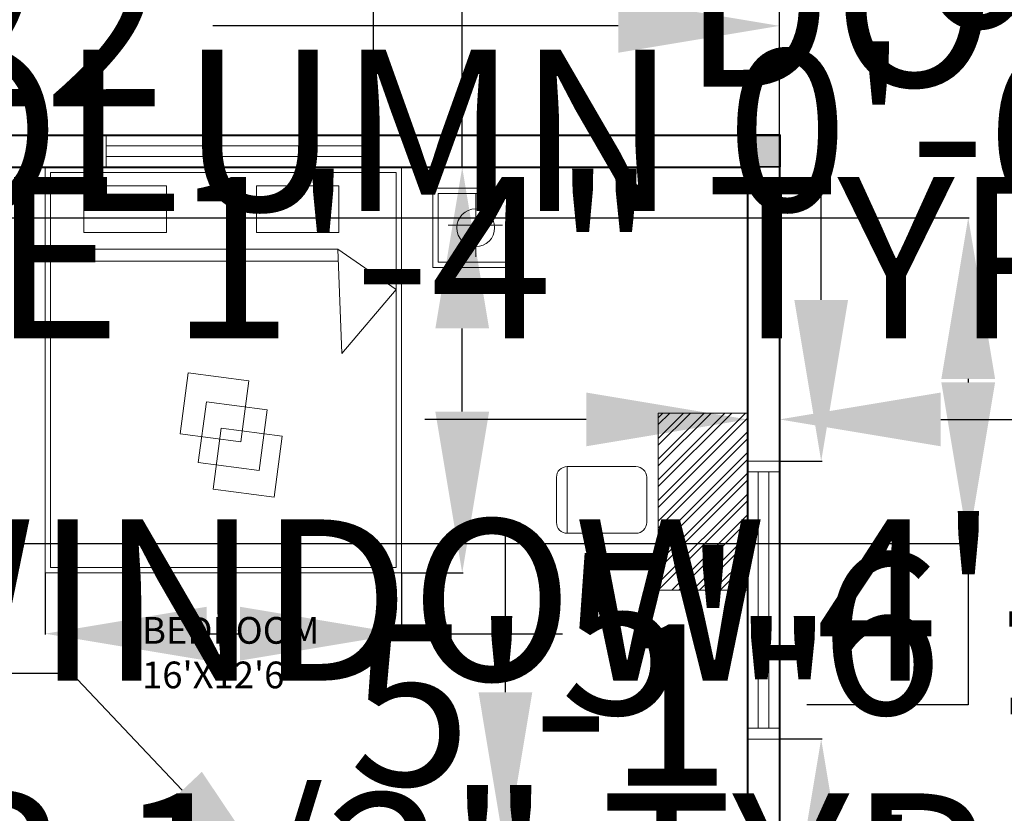
# Model space of a CAD drawing. Units: inches. Extents: x 7323 to 9737, y 2037 to 3322.
# Tile 15 of 19: x 9130 to 9314, y 2560 to 2709. Entities that reach past the tile are written whole.
import ezdxf

# ---------------------------------------------------------------- set-up
doc = ezdxf.new("R2010")
doc.units = ezdxf.units.IN
doc.header["$MEASUREMENT"] = 0
for name, color, linetype, lineweight in [('A-ANNO-DIMS', 2, 'Continuous', 18), ('A-AREA-IDEN', 7, 'Continuous', 18), ('A-COLS', 1, 'Continuous', 35), ('A-FURN', 8, 'Continuous', 18), ('A-FURN-PATT', 252, 'Continuous', 13), ('A-GLAZ', 4, 'Continuous', 18), ('A-WALL', 7, 'Continuous', 40)]:
    doc.layers.add(name, color=color, linetype=linetype, lineweight=lineweight)
doc.layers.add('A-COLS-PATT', color=18, linetype='Continuous', lineweight=13, true_color=0x000000)
doc.styles.get("Standard").update_dxf_attribs({"font": 'arial.ttf'})
doc.dimstyles.get("Standard").update_dxf_attribs({"dimtxt": 30.18, "dimasz": 30.18, "dimexe": 0.18, "dimexo": 0.0625, "dimgap": 0.09, "dimtad": 0, "dimtih": 1, "dimtoh": 1, "dimdec": 0, "dimzin": 0, "dimdsep": 46, "dimlunit": 3, "dimtxsty": 'Standard', "dimcen": 0.09, "dimadec": 0, "dimazin": 0, "dimtfac": 1, "dimtdec": 0, "dimtofl": 0, "dimtmove": 0, "dimatfit": 3, "dimfxl": 1, "dimtolj": 1, "dimtzin": 0, "dimarcsym": 0})

# ---------------------------------------------------------------- blocks, each defined once
blk = doc.blocks.new('*D10')
at = {"layer": 'A-ANNO-DIMS', "color": 0, "lineweight": -2, "transparency": 16777216}
for p, q in [((9007.95, 2687.36), (9007.95, 2707.94)), ((9038.13, 2707.76), (9113.99, 2707.76)), ((9241.77, 2707.76), (9165.9, 2707.76)), ((9271.95, 2687.36), (9271.95, 2707.94))]:
    blk.add_line(p, q, dxfattribs=at)
at = {"layer": 'A-ANNO-DIMS', "color": 0, "transparency": 16777216}
for points in [[(9038.13, 2712.79), (9038.13, 2702.73), (9007.95, 2707.76)], [(9241.77, 2712.79), (9241.77, 2702.73), (9271.95, 2707.76)]]:
    blk.add_solid(points, dxfattribs=at)
at = {"layer": 'Defpoints', "color": 0, "transparency": 16777216}
for p in [(9271.95, 2707.76), (9007.95, 2687.3), (9271.95, 2687.3)]:
    blk.add_point(p, dxfattribs=at)
at = {"layer": 'A-ANNO-DIMS', "color": 0, "transparency": 16777216, "insert": (9139.95, 2707.76), "char_height": 30.18, "attachment_point": 5}
blk.add_mtext("\\A1;22'", dxfattribs=at)
blk = doc.blocks.new('WIN-48')
for p, q in [((0, 0), (0, 6)), ((2, 0), (2, 6)), ((50, 0), (50, 6)), ((52, 0), (52, 6)), ((2, 4), (50, 4)), ((2, 2), (50, 2))]:
    blk.add_line(p, q)
blk = doc.blocks.new('BED-DOUBLE-REAR')
for p, q in [((1, 60.58), (54.75, 60.58)), ((54.75, 60.58), (65.65, 53.04)), ((55.5, 41.06), (54.75, 60.58)), ((54.83, 58.32), (1, 58.32)), ((65.65, 53.04), (55.5, 41.06))]:
    blk.add_line(p, q)
for points in [[(0, 75.91), (66.65, 75.91), (66.65, 0), (0, 0)], [(1, 74.91), (65.65, 74.91), (65.65, 1), (1, 1)], [(7.24, 72.42), (22.67, 72.42), (22.67, 63.7), (7.24, 63.7)], [(39.52, 72.42), (54.95, 72.42), (54.95, 63.7), (39.52, 63.7)], [(36.59, 24.55), (38.1, 35.92), (26.73, 37.42), (25.22, 26.05)], [(40.02, 19.16), (41.52, 30.53), (30.15, 32.04), (28.64, 20.66)], [(42.82, 14.19), (44.32, 25.56), (32.95, 27.06), (31.44, 15.69)]]:
    blk.add_lwpolyline(points, close=True)
blk = doc.blocks.new('BEDSIDE-TABLE-LARGE')
for p, q in [((8.01, 13.84), (8.01, 1.98)), ((2.84, 7.91), (13.05, 7.91))]:
    blk.add_line(p, q)
for points in [[(0, 14.84), (16.03, 14.84), (16.03, 0), (0, 0)], [(1, 13.84), (15.03, 13.84), (15.03, 1), (1, 1)]]:
    blk.add_lwpolyline(points, close=True)
blk.add_circle((8.01, 7.42), 3.54)
blk = doc.blocks.new('COL-PLAN-6IN')
blk.add_lwpolyline([(0, 6), (0, 6), (6.06, 6), (6.06, 6), (6.06, 0), (6.06, 0), (0, 0), (0, 0)], close=True)
blk = doc.blocks.new('*D35')
at = {"layer": 'A-ANNO-DIMS', "color": 0, "lineweight": -2, "transparency": 16777216}
for p, q in [((8977.7, 2688.2), (8947.52, 2688.2)), ((9007.88, 2687.36), (9007.88, 2688.38)), ((9013.95, 2687.36), (9013.95, 2688.38)), ((9044.13, 2688.2), (9074.31, 2688.2))]:
    blk.add_line(p, q, dxfattribs=at)
at = {"layer": 'A-ANNO-DIMS', "color": 0, "transparency": 16777216}
for points in [[(8977.7, 2693.23), (8977.7, 2683.17), (9007.88, 2688.2)], [(9044.13, 2693.23), (9044.13, 2683.17), (9013.95, 2688.2)]]:
    blk.add_solid(points, dxfattribs=at)
at = {"layer": 'Defpoints', "color": 0, "transparency": 16777216}
for p in [(9007.88, 2687.3), (9013.95, 2688.2), (9013.95, 2687.3)]:
    blk.add_point(p, dxfattribs=at)
at = {"layer": 'A-ANNO-DIMS', "color": 0, "transparency": 16777216, "insert": (9263.41, 2688.2), "char_height": 30.18, "attachment_point": 5}
blk.add_mtext('\\A1;COLUMN 0\'-6" TYP.', dxfattribs=at)
blk = doc.blocks.new('*D36')
at = {"layer": 'A-ANNO-DIMS', "color": 0, "lineweight": -2, "transparency": 16777216}
for p, q in [((9006.97, 2717.48), (9006.97, 2747.66)), ((9006.97, 2747.66), (9037.15, 2747.66)), ((9007.82, 2687.3), (9006.79, 2687.3)), ((9007.82, 2681.3), (9006.79, 2681.3)), ((9006.97, 2651.12), (9006.97, 2620.94))]:
    blk.add_line(p, q, dxfattribs=at)
at = {"layer": 'A-ANNO-DIMS', "color": 0, "transparency": 16777216}
for points in [[(9001.94, 2717.48), (9012, 2717.48), (9006.97, 2687.3)], [(9001.94, 2651.12), (9012, 2651.12), (9006.97, 2681.3)]]:
    blk.add_solid(points, dxfattribs=at)
at = {"layer": 'Defpoints', "color": 0, "transparency": 16777216}
for p in [(9006.97, 2687.3), (9007.88, 2687.3), (9007.88, 2681.3)]:
    blk.add_point(p, dxfattribs=at)
at = {"layer": 'A-ANNO-DIMS', "color": 0, "transparency": 16777216, "insert": (9129.22, 2747.66), "char_height": 30.18, "attachment_point": 5}
blk.add_mtext('\\A1;0\'-6" TYP.', dxfattribs=at)
blk = doc.blocks.new('*D37')
at = {"layer": 'A-ANNO-DIMS', "color": 0, "lineweight": -2, "transparency": 16777216}
for p, q in [((9279.75, 2656.48), (9279.75, 2686.66)), ((9272.01, 2626.3), (9279.93, 2626.3)), ((9272.01, 2574.3), (9279.93, 2574.3)), ((9279.75, 2544.12), (9279.75, 2513.94))]:
    blk.add_line(p, q, dxfattribs=at)
at = {"layer": 'A-ANNO-DIMS', "color": 0, "transparency": 16777216}
for points in [[(9274.72, 2656.48), (9284.78, 2656.48), (9279.75, 2626.3)], [(9274.72, 2544.12), (9284.78, 2544.12), (9279.75, 2574.3)]]:
    blk.add_solid(points, dxfattribs=at)
at = {"layer": 'Defpoints', "color": 0, "transparency": 16777216}
for p in [(9271.95, 2626.3), (9271.95, 2574.3), (9279.75, 2574.3)]:
    blk.add_point(p, dxfattribs=at)
at = {"layer": 'A-ANNO-DIMS', "color": 0, "transparency": 16777216, "insert": (9279.75, 2600.3), "char_height": 30.18, "attachment_point": 5}
blk.add_mtext('\\A1;WINDOW 4\'-4" TYP.', dxfattribs=at)
blk = doc.blocks.new('*D38')
at = {"layer": 'A-ANNO-DIMS', "color": 0, "lineweight": -2, "transparency": 16777216}
for p, q in [((9235.77, 2634.1), (9205.59, 2634.1)), ((9265.95, 2626.36), (9265.95, 2634.28)), ((9271.95, 2626.36), (9271.95, 2634.28)), ((9302.13, 2634.1), (9332.31, 2634.1))]:
    blk.add_line(p, q, dxfattribs=at)
at = {"layer": 'A-ANNO-DIMS', "color": 0, "transparency": 16777216}
for points in [[(9235.77, 2639.13), (9235.77, 2629.07), (9265.95, 2634.1)], [(9302.13, 2639.13), (9302.13, 2629.07), (9271.95, 2634.1)]]:
    blk.add_solid(points, dxfattribs=at)
at = {"layer": 'Defpoints', "color": 0, "transparency": 16777216}
for p in [(9271.95, 2634.1), (9265.95, 2626.3), (9271.95, 2626.3)]:
    blk.add_point(p, dxfattribs=at)
at = {"layer": 'A-ANNO-DIMS', "color": 0, "transparency": 16777216, "insert": (9424.38, 2634.1), "char_height": 30.18, "attachment_point": 5}
blk.add_mtext('\\A1;0\'-6" TYP.', dxfattribs=at)
blk = doc.blocks.new('*D39')
at = {"layer": 'A-ANNO-DIMS', "color": 0, "lineweight": -2, "transparency": 16777216}
for p, q in [((8647.94, 2549.03), (8617.76, 2549.03)), ((8678.12, 2543.2), (8678.12, 2549.21)), ((8717.39, 2543.2), (8717.39, 2549.21)), ((8747.57, 2549.03), (8777.75, 2549.03))]:
    blk.add_line(p, q, dxfattribs=at)
at = {"layer": 'A-ANNO-DIMS', "color": 0, "transparency": 16777216}
for points in [[(8647.94, 2554.06), (8647.94, 2544), (8678.12, 2549.03)], [(8747.57, 2554.06), (8747.57, 2544), (8717.39, 2549.03)]]:
    blk.add_solid(points, dxfattribs=at)
at = {"layer": 'Defpoints', "color": 0, "transparency": 16777216}
for p in [(8717.39, 2549.03), (8678.12, 2543.14), (8717.39, 2543.14)]:
    blk.add_point(p, dxfattribs=at)
at = {"layer": 'A-ANNO-DIMS', "color": 0, "transparency": 16777216, "insert": (9057.19, 2549.03), "char_height": 30.18, "attachment_point": 5}
blk.add_mtext('\\A1;SINGLE DOOR 3\'-3 1/2" TYP.', dxfattribs=at)
blk = doc.blocks.new('*D45')
at = {"layer": 'A-ANNO-DIMS', "color": 0, "lineweight": -2, "transparency": 16777216}
for p, q in [((8725.79, 2664.36), (8695.61, 2664.36)), ((8755.97, 2662.02), (8755.97, 2664.54)), ((8772, 2662.02), (8772, 2664.54)), ((8802.18, 2664.36), (8832.36, 2664.36))]:
    blk.add_line(p, q, dxfattribs=at)
at = {"layer": 'A-ANNO-DIMS', "color": 0, "transparency": 16777216}
for points in [[(8725.79, 2669.39), (8725.79, 2659.33), (8755.97, 2664.36)], [(8802.18, 2669.39), (8802.18, 2659.33), (8772, 2664.36)]]:
    blk.add_solid(points, dxfattribs=at)
at = {"layer": 'Defpoints', "color": 0, "transparency": 16777216}
for p in [(8772, 2664.36), (8755.97, 2661.96), (8772, 2661.96)]:
    blk.add_point(p, dxfattribs=at)
at = {"layer": 'A-ANNO-DIMS', "color": 0, "transparency": 16777216, "insert": (9094.8, 2664.36), "char_height": 30.18, "attachment_point": 5}
blk.add_mtext('\\A1;BEDSIDE TABLE 1\'-4" TYP.', dxfattribs=at)
blk = doc.blocks.new('*D51')
at = {"layer": 'A-ANNO-DIMS', "color": 0, "lineweight": -2, "transparency": 16777216}
for p, q in [((9130.95, 2513.23), (9130.95, 2501.42)), ((9208.95, 2513.23), (9208.95, 2501.42)), ((9161.13, 2501.6), (9178.77, 2501.6)), ((9208.95, 2501.6), (9239.13, 2501.6))]:
    blk.add_line(p, q, dxfattribs=at)
at = {"layer": 'A-ANNO-DIMS', "color": 0, "transparency": 16777216}
for points in [[(9161.13, 2506.63), (9161.13, 2496.57), (9130.95, 2501.6)], [(9178.77, 2506.63), (9178.77, 2496.57), (9208.95, 2501.6)]]:
    blk.add_solid(points, dxfattribs=at)
at = {"layer": 'Defpoints', "color": 0, "transparency": 16777216}
for p in [(9130.95, 2513.3), (9208.95, 2513.3), (9208.95, 2501.6)]:
    blk.add_point(p, dxfattribs=at)
at = {"layer": 'A-ANNO-DIMS', "color": 0, "transparency": 16777216, "insert": (9492.09, 2501.6), "char_height": 30.18, "attachment_point": 5}
blk.add_mtext('\\A1;DOUBLE DOOR 6\'-6" TYP.', dxfattribs=at)
blk = doc.blocks.new('*D52')
at = {"layer": 'A-ANNO-DIMS', "color": 0, "lineweight": -2, "transparency": 16777216}
for p, q in [((9220.65, 2583.03), (9220.65, 2613.21)), ((9209.01, 2552.85), (9220.83, 2552.85)), ((9209.01, 2513.3), (9220.83, 2513.3)), ((9220.65, 2483.12), (9220.65, 2452.94))]:
    blk.add_line(p, q, dxfattribs=at)
at = {"layer": 'A-ANNO-DIMS', "color": 0, "transparency": 16777216}
for points in [[(9215.62, 2583.03), (9225.68, 2583.03), (9220.65, 2552.85)], [(9215.62, 2483.12), (9225.68, 2483.12), (9220.65, 2513.3)]]:
    blk.add_solid(points, dxfattribs=at)
at = {"layer": 'Defpoints', "color": 0, "transparency": 16777216}
for p in [(9208.95, 2552.85), (9220.65, 2552.85), (9208.95, 2513.3)]:
    blk.add_point(p, dxfattribs=at)
at = {"layer": 'A-ANNO-DIMS', "color": 0, "transparency": 16777216, "insert": (9220.65, 2533.07), "char_height": 30.18, "attachment_point": 5}
blk.add_mtext('\\A1;3\'-3 1/2" TYP.', dxfattribs=at)
blk = doc.blocks.new('*D53')
at = {"layer": 'A-ANNO-DIMS', "color": 0, "lineweight": -2, "transparency": 16777216}
for p, q in [((8826.85, 2511.06), (8796.67, 2511.06)), ((8857.03, 2503.93), (8857.03, 2511.24)), ((8905.03, 2503.93), (8905.03, 2511.24)), ((8935.21, 2511.06), (8965.39, 2511.06))]:
    blk.add_line(p, q, dxfattribs=at)
at = {"layer": 'A-ANNO-DIMS', "color": 0, "transparency": 16777216}
for points in [[(8826.85, 2516.09), (8826.85, 2506.03), (8857.03, 2511.06)], [(8935.21, 2516.09), (8935.21, 2506.03), (8905.03, 2511.06)]]:
    blk.add_solid(points, dxfattribs=at)
at = {"layer": 'Defpoints', "color": 0, "transparency": 16777216}
for p in [(8905.03, 2511.06), (8857.03, 2503.86), (8905.03, 2503.86)]:
    blk.add_point(p, dxfattribs=at)
at = {"layer": 'A-ANNO-DIMS', "color": 0, "transparency": 16777216, "insert": (9261.3, 2511.06), "char_height": 30.18, "attachment_point": 5}
blk.add_mtext('\\A1;INTERIOR WINDOW 4\'-0" TYP.', dxfattribs=at)
blk = doc.blocks.new('*D59')
at = {"layer": 'A-ANNO-DIMS', "color": 0, "lineweight": -2, "transparency": 16777216}
for p, q in [((9064.67, 2473.96), (9064.67, 2467.95)), ((9103.95, 2473.96), (9103.95, 2467.95)), ((9034.49, 2468.13), (9004.31, 2468.13)), ((9134.13, 2468.13), (9164.31, 2468.13))]:
    blk.add_line(p, q, dxfattribs=at)
at = {"layer": 'A-ANNO-DIMS', "color": 0, "transparency": 16777216}
for points in [[(9034.49, 2473.16), (9034.49, 2463.1), (9064.67, 2468.13)], [(9134.13, 2473.16), (9134.13, 2463.1), (9103.95, 2468.13)]]:
    blk.add_solid(points, dxfattribs=at)
at = {"layer": 'Defpoints', "color": 0, "transparency": 16777216}
for p in [(9064.67, 2474.02), (9103.95, 2474.02), (9103.95, 2468.13)]:
    blk.add_point(p, dxfattribs=at)
at = {"layer": 'A-ANNO-DIMS', "color": 0, "transparency": 16777216, "insert": (9458.35, 2468.13), "char_height": 30.18, "attachment_point": 5}
blk.add_mtext('\\A1;KITCHEN DOOR 3\'-3 1/2" TYP.', dxfattribs=at)
blk = doc.blocks.new('*D60')
at = {"layer": 'A-ANNO-DIMS', "color": 0, "lineweight": -2, "transparency": 16777216}
for p, q in [((9109.84, 2540.48), (9109.84, 2570.66)), ((9104.01, 2510.3), (9110.02, 2510.3)), ((9104.01, 2474.02), (9110.02, 2474.02)), ((9109.84, 2443.84), (9109.84, 2413.66))]:
    blk.add_line(p, q, dxfattribs=at)
at = {"layer": 'A-ANNO-DIMS', "color": 0, "transparency": 16777216}
for points in [[(9104.81, 2540.48), (9114.87, 2540.48), (9109.84, 2510.3)], [(9104.81, 2443.84), (9114.87, 2443.84), (9109.84, 2474.02)]]:
    blk.add_solid(points, dxfattribs=at)
at = {"layer": 'Defpoints', "color": 0, "transparency": 16777216}
for p in [(9103.95, 2510.3), (9109.84, 2510.3), (9103.95, 2474.02)]:
    blk.add_point(p, dxfattribs=at)
at = {"layer": 'A-ANNO-DIMS', "color": 0, "transparency": 16777216, "insert": (9109.84, 2492.16), "char_height": 30.18, "attachment_point": 5}
blk.add_mtext('\\A1;3\'-0 1/2" TYP.', dxfattribs=at)
blk = doc.blocks.new('*D61')
at = {"layer": 'A-ANNO-DIMS', "color": 0, "lineweight": -2, "transparency": 16777216}
for p, q in [((9212.57, 2681.3), (9212.57, 2711.48)), ((9212.57, 2711.48), (9242.75, 2711.48)), ((9201.24, 2681.3), (9212.75, 2681.3)), ((9212.57, 2635.56), (9212.57, 2651.12)), ((9201.24, 2605.38), (9212.75, 2605.38))]:
    blk.add_line(p, q, dxfattribs=at)
at = {"layer": 'A-ANNO-DIMS', "color": 0, "transparency": 16777216}
for points in [[(9207.54, 2651.12), (9217.6, 2651.12), (9212.57, 2681.3)], [(9207.54, 2635.56), (9217.6, 2635.56), (9212.57, 2605.38)]]:
    blk.add_solid(points, dxfattribs=at)
at = {"layer": 'Defpoints', "color": 0, "transparency": 16777216}
for p in [(9201.18, 2681.3), (9212.57, 2681.3), (9201.18, 2605.38)]:
    blk.add_point(p, dxfattribs=at)
at = {"layer": 'A-ANNO-DIMS', "color": 0, "transparency": 16777216, "insert": (9475.82, 2711.48), "char_height": 30.18, "attachment_point": 5}
blk.add_mtext('\\A1;DOUBLE BED 6\'-4" TYP.', dxfattribs=at)
blk = doc.blocks.new('*D62')
at = {"layer": 'A-ANNO-DIMS', "color": 0, "lineweight": -2, "transparency": 16777216}
for p, q in [((9134.53, 2605.32), (9134.53, 2593.82)), ((9201.18, 2605.32), (9201.18, 2593.82)), ((9164.71, 2594), (9171, 2594)), ((9201.18, 2594), (9231.36, 2594))]:
    blk.add_line(p, q, dxfattribs=at)
at = {"layer": 'A-ANNO-DIMS', "color": 0, "transparency": 16777216}
for points in [[(9164.71, 2599.03), (9164.71, 2588.97), (9134.53, 2594)], [(9171, 2599.03), (9171, 2588.97), (9201.18, 2594)]]:
    blk.add_solid(points, dxfattribs=at)
at = {"layer": 'Defpoints', "color": 0, "transparency": 16777216}
for p in [(9134.53, 2605.38), (9201.18, 2605.38), (9201.18, 2594)]:
    blk.add_point(p, dxfattribs=at)
at = {"layer": 'A-ANNO-DIMS', "color": 0, "transparency": 16777216, "insert": (9358.59, 2594), "char_height": 30.18, "attachment_point": 5}
blk.add_mtext('\\A1;5\'-6 1/2" TYP.', dxfattribs=at)
blk = doc.blocks.new('*D63')
at = {"layer": 'A-ANNO-DIMS', "color": 0, "lineweight": -2, "transparency": 16777216}
for p, q in [((8744.72, 2466.22), (8744.72, 2496.4)), ((8744.72, 2496.4), (8774.9, 2496.4)), ((8741.46, 2436.04), (8744.9, 2436.04)), ((8741.46, 2413.86), (8744.9, 2413.86)), ((8744.72, 2383.68), (8744.72, 2353.5))]:
    blk.add_line(p, q, dxfattribs=at)
at = {"layer": 'A-ANNO-DIMS', "color": 0, "transparency": 16777216}
for points in [[(8739.69, 2466.22), (8749.75, 2466.22), (8744.72, 2436.04)], [(8739.69, 2383.68), (8749.75, 2383.68), (8744.72, 2413.86)]]:
    blk.add_solid(points, dxfattribs=at)
at = {"layer": 'Defpoints', "color": 0, "transparency": 16777216}
for p in [(8741.39, 2436.04), (8744.72, 2436.04), (8741.39, 2413.86)]:
    blk.add_point(p, dxfattribs=at)
at = {"layer": 'A-ANNO-DIMS', "color": 0, "transparency": 16777216, "insert": (9003.76, 2496.4), "char_height": 30.18, "attachment_point": 5}
blk.add_mtext('\\A1;APPLIANCE 1\'-10" TYP.', dxfattribs=at)
blk = doc.blocks.new('*D65')
at = {"layer": 'A-ANNO-DIMS', "color": 0, "lineweight": -2, "transparency": 16777216}
for p, q in [((9024.02, 2513.3), (9024.02, 2543.48)), ((9024.02, 2543.48), (9054.2, 2543.48)), ((9036.56, 2513.3), (9023.84, 2513.3)), ((9024.02, 2459.48), (9024.02, 2483.12)), ((9036.56, 2429.3), (9023.84, 2429.3))]:
    blk.add_line(p, q, dxfattribs=at)
at = {"layer": 'A-ANNO-DIMS', "color": 0, "transparency": 16777216}
for points in [[(9018.99, 2483.12), (9029.05, 2483.12), (9024.02, 2513.3)], [(9018.99, 2459.48), (9029.05, 2459.48), (9024.02, 2429.3)]]:
    blk.add_solid(points, dxfattribs=at)
at = {"layer": 'Defpoints', "color": 0, "transparency": 16777216}
for p in [(9024.02, 2513.3), (9036.62, 2513.3), (9036.62, 2429.3)]:
    blk.add_point(p, dxfattribs=at)
at = {"layer": 'A-ANNO-DIMS', "color": 0, "transparency": 16777216, "insert": (9256.18, 2543.48), "char_height": 30.18, "attachment_point": 5}
blk.add_mtext('\\A1;COUNTER 7\'-0" TYP.', dxfattribs=at)
blk = doc.blocks.new('*D66')
at = {"layer": 'A-ANNO-DIMS', "color": 0, "lineweight": -2, "transparency": 16777216}
for p, q in [((9006.44, 2525.9), (8976.26, 2525.9)), ((9036.62, 2513.36), (9036.62, 2526.08)), ((9075.95, 2513.36), (9075.95, 2526.08)), ((9106.13, 2525.9), (9136.31, 2525.9))]:
    blk.add_line(p, q, dxfattribs=at)
at = {"layer": 'A-ANNO-DIMS', "color": 0, "transparency": 16777216}
for points in [[(9006.44, 2530.93), (9006.44, 2520.87), (9036.62, 2525.9)], [(9106.13, 2530.93), (9106.13, 2520.87), (9075.95, 2525.9)]]:
    blk.add_solid(points, dxfattribs=at)
at = {"layer": 'Defpoints', "color": 0, "transparency": 16777216}
for p in [(9075.95, 2525.9), (9036.62, 2513.3), (9075.95, 2513.3)]:
    blk.add_point(p, dxfattribs=at)
at = {"layer": 'A-ANNO-DIMS', "color": 0, "transparency": 16777216, "insert": (9263.53, 2525.9), "char_height": 30.18, "attachment_point": 5}
blk.add_mtext('\\A1;3\'-3 1/2" TYP.', dxfattribs=at)
blk = doc.blocks.new('*D69')
at = {"layer": 'A-ANNO-DIMS', "color": 0, "lineweight": -2, "transparency": 16777216}
for p, q in [((8836.58, 2472.89), (8836.58, 2503.07)), ((8836.58, 2503.07), (8866.76, 2503.07)), ((8839.88, 2442.71), (8836.4, 2442.71)), ((8839.88, 2420.33), (8836.4, 2420.33)), ((8836.58, 2390.15), (8836.58, 2359.97))]:
    blk.add_line(p, q, dxfattribs=at)
at = {"layer": 'A-ANNO-DIMS', "color": 0, "transparency": 16777216}
for points in [[(8831.55, 2472.89), (8841.61, 2472.89), (8836.58, 2442.71)], [(8831.55, 2390.15), (8841.61, 2390.15), (8836.58, 2420.33)]]:
    blk.add_solid(points, dxfattribs=at)
at = {"layer": 'Defpoints', "color": 0, "transparency": 16777216}
for p in [(8836.58, 2442.71), (8839.94, 2442.71), (8839.94, 2420.33)]:
    blk.add_point(p, dxfattribs=at)
at = {"layer": 'A-ANNO-DIMS', "color": 0, "transparency": 16777216, "insert": (9169.54, 2503.07), "char_height": 30.18, "attachment_point": 5}
blk.add_mtext('\\A1;COFFEE TABLE 1\'-10 1/2" TYP.', dxfattribs=at)
blk = doc.blocks.new('*D114')
at = {"layer": 'A-ANNO-DIMS', "color": 0, "lineweight": -2, "transparency": 16777216}
for p, q in [((8915.46, 2671.86), (9307.45, 2671.86)), ((9307.27, 2641.68), (9307.27, 2641.04)), ((8915.46, 2610.86), (9307.45, 2610.86)), ((9307.27, 2610.86), (9307.27, 2580.68)), ((9307.27, 2580.68), (9277.09, 2580.68))]:
    blk.add_line(p, q, dxfattribs=at)
at = {"layer": 'A-ANNO-DIMS', "color": 0, "transparency": 16777216}
for points in [[(9302.24, 2641.68), (9312.3, 2641.68), (9307.27, 2671.86)], [(9302.24, 2641.04), (9312.3, 2641.04), (9307.27, 2610.86)]]:
    blk.add_solid(points, dxfattribs=at)
at = {"layer": 'Defpoints', "color": 0, "transparency": 16777216}
for p in [(8915.39, 2671.86), (8915.39, 2610.86), (9307.27, 2610.86)]:
    blk.add_point(p, dxfattribs=at)
at = {"layer": 'A-ANNO-DIMS', "color": 0, "transparency": 16777216, "insert": (9236.89, 2580.68), "char_height": 30.18, "attachment_point": 5}
blk.add_mtext('\\A1;5\'-1"', dxfattribs=at)
blk = doc.blocks.new('*D123')
at = {"layer": 'A-ANNO-DIMS', "color": 0, "lineweight": -2, "transparency": 16777216}
for p, q in [((9195.95, 2687.36), (9195.95, 2722.73)), ((9226.13, 2722.55), (9241.77, 2722.55)), ((9271.95, 2687.36), (9271.95, 2722.73)), ((9271.95, 2722.55), (9302.13, 2722.55))]:
    blk.add_line(p, q, dxfattribs=at)
at = {"layer": 'A-ANNO-DIMS', "color": 0, "transparency": 16777216}
for points in [[(9226.13, 2727.58), (9226.13, 2717.52), (9195.95, 2722.55)], [(9241.77, 2727.58), (9241.77, 2717.52), (9271.95, 2722.55)]]:
    blk.add_solid(points, dxfattribs=at)
at = {"layer": 'Defpoints', "color": 0, "transparency": 16777216}
for p in [(9271.95, 2722.55), (9195.95, 2687.3), (9271.95, 2687.3)]:
    blk.add_point(p, dxfattribs=at)
at = {"layer": 'A-ANNO-DIMS', "color": 0, "transparency": 16777216, "insert": (9342.41, 2722.55), "char_height": 30.18, "attachment_point": 5}
blk.add_mtext('\\A1;6\'-4"', dxfattribs=at)
blk = doc.blocks.new('*D126')
at = {"layer": 'A-ANNO-DIMS', "color": 0, "lineweight": -2, "transparency": 16777216}
for p, q in [((9109.28, 2586.63), (9139.46, 2586.63)), ((9139.46, 2586.63), (9160.18, 2564.69)), ((9204.86, 2517.3), (9205.04, 2517.3)), ((9204.95, 2517.21), (9204.95, 2517.39))]:
    blk.add_line(p, q, dxfattribs=at)
at = {"layer": 'A-ANNO-DIMS', "color": 0, "transparency": 16777216}
blk.add_solid([(9163.84, 2568.15), (9156.52, 2561.24), (9180.9, 2542.75)], dxfattribs=at)
at = {"layer": 'Defpoints', "color": 0, "transparency": 16777216}
for p in [(9180.9, 2542.75), (9204.95, 2517.3)]:
    blk.add_point(p, dxfattribs=at)
at = {"layer": 'A-ANNO-DIMS', "color": 0, "transparency": 16777216, "insert": (9009.88, 2586.63), "char_height": 30.18, "attachment_point": 5}
blk.add_mtext('\\A1;4X R2\'-11"', dxfattribs=at)

msp = doc.modelspace()

# ---------------------------------------------------------------- hatches: boundary and pattern name
at = {"layer": 'A-COLS-PATT'}
h = msp.add_hatch(color=256, dxfattribs=at)
h.dxf.hatch_style = 1
h.paths.add_polyline_path([(8915.39, 2189.86), (8908.77, 2189.86), (8908.77, 2183.86), (8915.39, 2183.86)])
h.paths.add_polyline_path([(8657.61, 2189.86), (8651.55, 2189.86), (8651.55, 2183.86), (8657.61, 2183.86)])
h.paths.add_polyline_path([(8814.13, 2189.86), (8807.39, 2189.86), (8807.39, 2183.86), (8814.13, 2183.86)])
h.paths.add_polyline_path([(8813.39, 2317.86), (8807.36, 2317.86), (8807.36, 2311.86), (8813.39, 2311.86)])
h.paths.add_polyline_path([(8915.34, 2313.13), (8909.39, 2313.13), (8909.39, 2307.13), (8915.34, 2307.13)])
h.paths.add_polyline_path([(8657.62, 2317.86), (8657.39, 2317.86), (8657.39, 2318.08), (8651.55, 2318.08), (8651.55, 2312.08), (8657.62, 2312.08)])
h.paths.add_polyline_path([(8915.39, 2671.84), (8909.37, 2671.84), (8909.37, 2665.86), (8909.39, 2665.86), (8915.39, 2665.84)])
h.paths.add_polyline_path([(8657.59, 2671.81), (8651.52, 2671.81), (8651.52, 2665.81), (8657.39, 2665.81), (8657.39, 2665.86)])
h.paths.add_polyline_path([(8915.28, 2503.94), (8909.39, 2503.94), (8909.39, 2503.86), (8909.22, 2497.94), (8915.28, 2497.94)])
h.paths.add_polyline_path([(8657.53, 2503.86), (8657.39, 2503.86), (8651.46, 2503.96), (8651.46, 2497.96), (8657.53, 2497.96)])
h.paths.add_polyline_path([(9014.24, 2519.3), (9013.95, 2519.3), (9008.18, 2519.31), (9008.18, 2513.31), (9014.24, 2513.31)])
h.paths.add_polyline_path([(9013.95, 2687.3), (9007.95, 2687.3), (9007.95, 2681.3), (9013.95, 2681.3)])
h.paths.add_polyline_path([(9271.95, 2687.3), (9266.01, 2687.3), (9266.01, 2681.35), (9271.95, 2681.35)])
h.paths.add_polyline_path([(9271.95, 2205.3), (9265.32, 2205.3), (9265.32, 2199.3), (9271.95, 2199.3)])
h.paths.add_polyline_path([(9170.68, 2205.3), (9163.95, 2205.3), (9163.95, 2199.3), (9170.68, 2199.3)])
h.paths.add_polyline_path([(9013.95, 2205.3), (9007.95, 2205.3), (9007.95, 2199.3), (9013.95, 2199.3)])
h.paths.add_polyline_path([(9271.95, 2519.51), (9265.95, 2519.51), (9265.95, 2519.3), (9265.93, 2513.51), (9271.95, 2513.51)])
h.paths.add_polyline_path([(9271.95, 2328.64), (9265.95, 2328.64), (9265.95, 2322.64), (9271.95, 2322.64)])
h.paths.add_polyline_path([(9014.35, 2333.3), (9013.95, 2333.3), (9013.95, 2333.58), (9008.29, 2333.58), (9008.29, 2327.58), (9014.35, 2327.58)])
at = {"layer": 'A-FURN-PATT'}
h = msp.add_hatch(dxfattribs=at)
h.set_pattern_fill('ANSI32', color=256, scale=7.3)
h.set_pattern_definition([(45, (1817.2537, -453.8612), (-1.9357048, 1.9357048), []), (45, (1818.5442, -453.8612), (-1.9357048, 1.9357048), [])])
h.paths.add_polyline_path([(9249.26, 2602.13), (9265.95, 2602.13), (9265.95, 2635.27), (9249.26, 2635.27)])

# ---------------------------------------------------------------- linework, layer by layer
at = {"layer": 'A-FURN'}
msp.add_line((9232.21, 2625.28), (9232.21, 2612.8), dxfattribs=at)
msp.add_lwpolyline([(9265.95, 2635.27), (9249.26, 2635.27), (9249.26, 2602.13), (9265.95, 2602.13)], close=True, dxfattribs=at)
msp.add_lwpolyline([(9230.21, 2623.28, -0.414214), (9232.21, 2625.28), (9245.09, 2625.28, -0.414214), (9247.09, 2623.28), (9247.09, 2614.8, -0.414214), (9245.09, 2612.8), (9232.21, 2612.8, -0.414214), (9230.21, 2614.8)], format="xyb", close=True, dxfattribs=at)
at = {"layer": 'A-WALL'}
for p, q in [((9007.95, 2687.3), (9271.95, 2687.3)), ((9271.95, 2687.3), (9271.95, 2199.3)), ((9073.95, 2681.3), (9265.95, 2681.3)), ((9265.95, 2681.3), (9265.95, 2519.3))]:
    msp.add_line(p, q, dxfattribs=at)

# ---------------------------------------------------------------- block references
at = {"layer": 'A-COLS'}
msp.add_blockref('COL-PLAN-6IN', (9266.01, 2681.35), dxfattribs=at)
at = {"layer": 'A-FURN'}
for name, p in [('BED-DOUBLE-REAR', (9134.53, 2605.38)), ('BEDSIDE-TABLE-LARGE', (9207.08, 2662.55))]:
    msp.add_blockref(name, p, dxfattribs=at)
at = {"layer": 'A-GLAZ'}
for p, rotation in [((9195.95, 2687.3), 180), ((9265.95, 2626.29), 270.000000000004)]:
    msp.add_blockref('WIN-48', p, dxfattribs=dict(at, rotation=rotation))

# ---------------------------------------------------------------- texts
at = {"layer": 'A-AREA-IDEN', "insert": (9152.65, 2597.12), "char_height": 5, "attachment_point": 1}
msp.add_mtext_dynamic_manual_height_columns('BEDROOM\\P16\'X12\'6"', width=44.1759, gutter_width=1, heights=[0], dxfattribs=at)

# ---------------------------------------------------------------- dimensions: what is measured, and where the dimension line sits
at = {"layer": 'A-ANNO-DIMS'}
for base, p1, p2, angle, text, picture, middle in [((9212.57, 2681.3), (9201.18, 2605.38), (9201.18, 2681.3), 90, 'DOUBLE BED <> TYP.', '*D61', (9475.82, 2711.48)), ((9006.97, 2687.3), (9007.88, 2681.3), (9007.88, 2687.3), 90, '<> TYP.', '*D36', (9129.22, 2747.66)), ((9279.75, 2574.3), (9271.95, 2626.3), (9271.95, 2574.3), 270, 'WINDOW <> TYP.', '*D37', (9279.75, 2600.3)), ((9271.95, 2634.1), (9265.95, 2626.3), (9271.95, 2626.3), 0, '<> TYP.', '*D38', (9424.38, 2634.1)), ((8836.58, 2442.71), (8839.94, 2420.33), (8839.94, 2442.71), 90, 'COFFEE TABLE <> TYP.', '*D69', (9169.54, 2503.07)), ((9024.02, 2513.3), (9036.62, 2429.3), (9036.62, 2513.3), 90, 'COUNTER <> TYP.', '*D65', (9256.18, 2543.48)), ((9220.6454, 2552.8475), (9208.9454, 2513.2952), (9208.9454, 2552.8475), 90, '<> TYP.', '*D52', (9220.6454, 2533.0713)), ((9109.84, 2510.3), (9103.95, 2474.02), (9103.95, 2510.3), 90, '<> TYP.', '*D60', (9109.84, 2492.16)), ((8744.72, 2436.04), (8741.39, 2413.86), (8741.39, 2436.04), 90, 'APPLIANCE <> TYP.', '*D63', (9003.76, 2496.4))]:
    dim = msp.add_linear_dim(base=base, p1=p1, p2=p2, angle=angle, text=text, dimstyle='Standard', override={"dimdec": 1, "dimlfac": 1, "dimrnd": 0, "dimzin": 1, "dimdsep": 46, "dimlunit": 4, "dimfrac": 2}, dxfattribs=at)
    dim.commit()
    dim.dimension.update_dxf_attribs({"geometry": picture, "text_midpoint": middle})
for base, p1, p2, text, picture, middle in [((8772, 2664.36), (8755.97, 2661.96), (8772, 2661.96), 'BEDSIDE TABLE <> TYP.', '*D45', (9094.8, 2664.36)), ((9013.95, 2688.2), (9007.88, 2687.3), (9013.95, 2687.3), 'COLUMN <> TYP.', '*D35', (9263.41, 2688.2)), ((8717.39, 2549.03), (8678.12, 2543.14), (8717.39, 2543.14), 'SINGLE DOOR <> TYP.', '*D39', (9057.19, 2549.03)), ((9201.1793, 2593.9956), (9134.5282, 2605.3825), (9201.1793, 2605.3825), '<> TYP.', '*D62', (9358.5924, 2593.9956)), ((8905.03, 2511.06), (8857.03, 2503.86), (8905.03, 2503.86), 'INTERIOR WINDOW <> TYP.', '*D53', (9261.3, 2511.06)), ((9208.95, 2501.6), (9130.95, 2513.3), (9208.95, 2513.3), 'DOUBLE DOOR <> TYP.', '*D51', (9492.09, 2501.6)), ((9075.95, 2525.9), (9036.62, 2513.3), (9075.95, 2513.3), '<> TYP.', '*D66', (9263.53, 2525.9)), ((9103.95, 2468.13), (9064.67, 2474.02), (9103.95, 2474.02), 'KITCHEN DOOR <> TYP.', '*D59', (9458.35, 2468.13))]:
    dim = msp.add_linear_dim(base=base, p1=p1, p2=p2, text=text, dimstyle='Standard', override={"dimdec": 1, "dimlfac": 1, "dimrnd": 0, "dimzin": 1, "dimdsep": 46, "dimlunit": 4, "dimfrac": 2}, dxfattribs=at)
    dim.commit()
    dim.dimension.update_dxf_attribs({"geometry": picture, "text_midpoint": middle})
for base, p1, override, picture, middle in [((9271.95, 2722.55), (9195.95, 2687.3), {"dimdec": 1, "dimlfac": 1, "dimrnd": 0, "dimzin": 1, "dimdsep": 46, "dimlunit": 4, "dimfrac": 2}, '*D123', (9342.41, 2722.55)), ((9271.95, 2707.76), (9007.95, 2687.3), {"dimclrd": 0, "dimclre": 0, "dimclrt": 0}, '*D10', (9139.95, 2707.76))]:
    dim = msp.add_linear_dim(base=base, p1=p1, p2=(9271.95, 2687.3), dimstyle='Standard', override=override, dxfattribs=at)
    dim.commit()
    dim.dimension.update_dxf_attribs({"geometry": picture, "text_midpoint": middle})
dim = msp.add_linear_dim(base=(9307.27, 2610.86), p1=(8915.39, 2671.86), p2=(8915.39, 2610.86), angle=90, dimstyle='Standard', override={"dimdec": 1, "dimlfac": 1, "dimrnd": 0, "dimzin": 1, "dimdsep": 46, "dimlunit": 4, "dimfrac": 2}, dxfattribs=at)
dim.commit()
dim.dimension.update_dxf_attribs({"geometry": '*D114', "text_midpoint": (9236.89, 2580.68)})
dim = msp.add_radius_dim(center=(9204.95, 2517.3), mpoint=(9180.9, 2542.75), text='4X <>', dimstyle='Standard', override={"dimdec": 1, "dimlfac": 1, "dimrnd": 0, "dimzin": 1, "dimdsep": 46, "dimlunit": 4, "dimfrac": 2}, dxfattribs=at)
dim.commit()
dim.dimension.update_dxf_attribs({"geometry": '*D126', "text_midpoint": (9009.88, 2586.63)})

doc.saveas('drawing.dxf')
